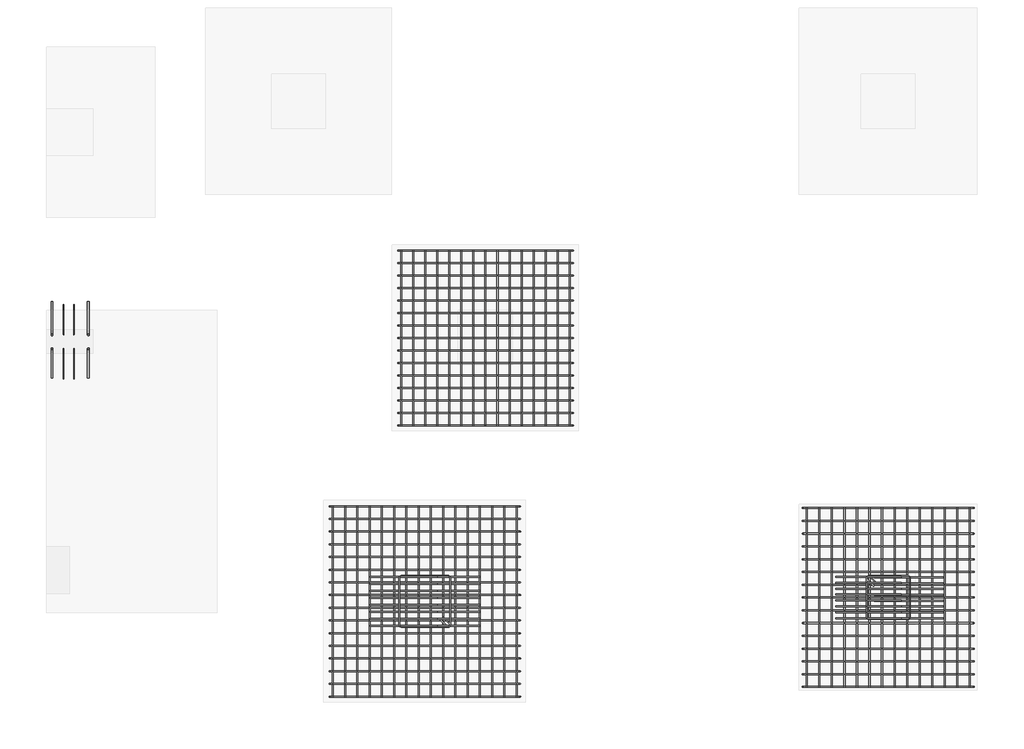
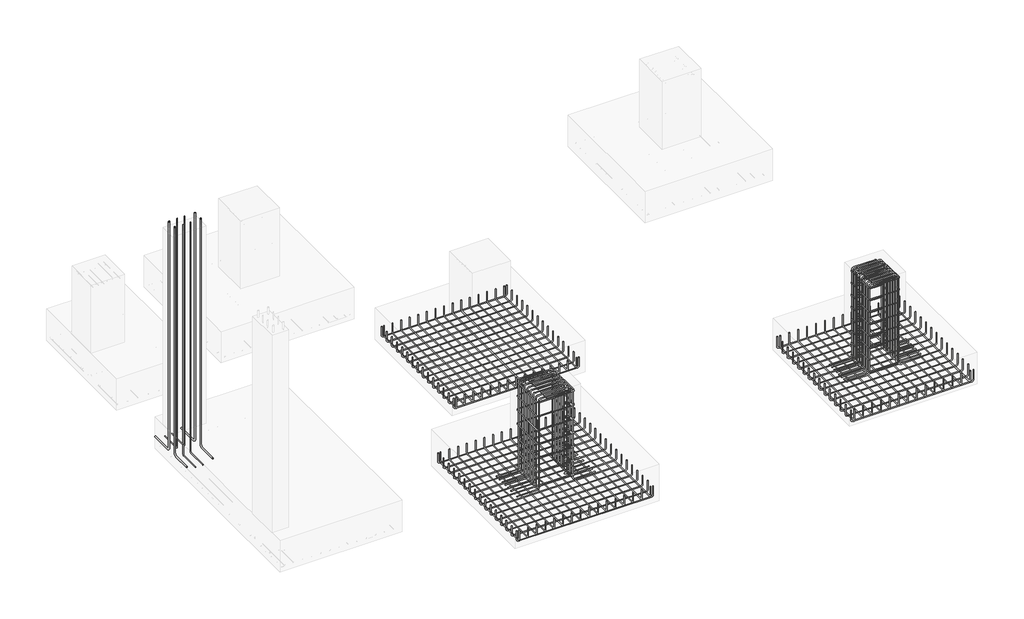
# One storey, part 4 of 6: 16 reinforcing bars.
"""IFC4 building model written with IfcOpenShell, lengths in millimetres."""

from ifc_helpers import new_model, si_unit, point, frame, origin, place, context, project, spatial, polyline, circle_curve, trimmed, segment, composite_curve, source, transform, mapped, element, save
from ifc_brep_helpers import swept_disk

model = new_model("IFC4")

# Units and contexts
model_context = context("Model", 3, world=origin())
ifc_project = project(units=[si_unit("LENGTHUNIT", "METRE", prefix="MILLI")], contexts=[model_context])

# Site, building, storey
site = spatial("IfcSite", under=ifc_project)
building = spatial("IfcBuilding", under=site)
storey = spatial("IfcBuildingStorey", under=building, Elevation=0.0)

# Reinforcing bars
placement = place(None, origin())
reinforcing_bar_shape = source(origin(), model_context, "Body", "SolidModel", [
    swept_disk(composite_curve([segment(polyline([(157700.823207, -99129.4007776, -254.8), (157700.823207, -99129.4007776, -397.2)]), True, "CONTINUOUS"), segment(trimmed(circle_curve(frame((157725.823207, -99129.4007776, -397.2), z_axis=(0.0, -1.0, 0.0), x_axis=(-25.0, 0.0, 0.0)), 25.0), [point((157700.823207, -99129.4007776, -397.2))], [point((157725.823207, -99129.4007776, -422.2))], True, "CARTESIAN"), True, "CONTINUOUS"), segment(polyline([(157725.823207, -99129.4007776, -422.2), (159358.423207, -99129.4007776, -422.2)]), True, "CONTINUOUS"), segment(trimmed(circle_curve(frame((159358.423207, -99129.4007776, -397.2), z_axis=(0.0, -1.0, 0.0), x_axis=(0.0, 0.0, -25.0)), 25.0), [point((159358.423207, -99129.4007776, -422.2))], [point((159383.423207, -99129.4007776, -397.2))], True, "CARTESIAN"), True, "CONTINUOUS"), segment(polyline([(159383.423207, -99129.4007776, -397.2), (159383.423207, -99129.4007776, -254.8)]), True, "CONTINUOUS")], self_intersect=False), 5.0),
])
element("IfcReinforcingBar", 1, at=placement, inside=storey, context=model_context, shape_type="MappedRepresentation", body=[
    mapped(reinforcing_bar_shape, transform((0.0, 0.0, 0.0), x_axis=(1.0, 0.0, 0.0), y_axis=(0.0, 1.0, 0.0), z_axis=(0.0, 0.0, 1.0))),
    mapped(reinforcing_bar_shape, transform((0.0, -125.6285714, 0.0), x_axis=(1.0, 0.0, 0.0), y_axis=(0.0, 1.0, 0.0), z_axis=(0.0, 0.0, 1.0))),
    mapped(reinforcing_bar_shape, transform((0.0, -251.2571429, 0.0), x_axis=(1.0, 0.0, 0.0), y_axis=(0.0, 1.0, 0.0), z_axis=(0.0, 0.0, 1.0))),
    mapped(reinforcing_bar_shape, transform((0.0, -376.8857143, 0.0), x_axis=(1.0, 0.0, 0.0), y_axis=(0.0, 1.0, 0.0), z_axis=(0.0, 0.0, 1.0))),
    mapped(reinforcing_bar_shape, transform((0.0, -502.5142857, 0.0), x_axis=(1.0, 0.0, 0.0), y_axis=(0.0, 1.0, 0.0), z_axis=(0.0, 0.0, 1.0))),
    mapped(reinforcing_bar_shape, transform((0.0, -628.1428571, 0.0), x_axis=(1.0, 0.0, 0.0), y_axis=(0.0, 1.0, 0.0), z_axis=(0.0, 0.0, 1.0))),
    mapped(reinforcing_bar_shape, transform((0.0, -753.7714286, 0.0), x_axis=(1.0, 0.0, 0.0), y_axis=(0.0, 1.0, 0.0), z_axis=(0.0, 0.0, 1.0))),
    mapped(reinforcing_bar_shape, transform((0.0, -879.4, 0.0), x_axis=(1.0, 0.0, 0.0), y_axis=(0.0, 1.0, 0.0), z_axis=(0.0, 0.0, 1.0))),
    mapped(reinforcing_bar_shape, transform((0.0, -1005.0285714, 0.0), x_axis=(1.0, 0.0, 0.0), y_axis=(0.0, 1.0, 0.0), z_axis=(0.0, 0.0, 1.0))),
    mapped(reinforcing_bar_shape, transform((0.0, -1130.6571429, 0.0), x_axis=(1.0, 0.0, 0.0), y_axis=(0.0, 1.0, 0.0), z_axis=(0.0, 0.0, 1.0))),
    mapped(reinforcing_bar_shape, transform((0.0, -1256.2857143, 0.0), x_axis=(1.0, 0.0, 0.0), y_axis=(0.0, 1.0, 0.0), z_axis=(0.0, 0.0, 1.0))),
    mapped(reinforcing_bar_shape, transform((0.0, -1381.9142857, 0.0), x_axis=(1.0, 0.0, 0.0), y_axis=(0.0, 1.0, 0.0), z_axis=(0.0, 0.0, 1.0))),
    mapped(reinforcing_bar_shape, transform((0.0, -1507.5428571, 0.0), x_axis=(1.0, 0.0, 0.0), y_axis=(0.0, 1.0, 0.0), z_axis=(0.0, 0.0, 1.0))),
    mapped(reinforcing_bar_shape, transform((0.0, -1633.1714286, 0.0), x_axis=(1.0, 0.0, 0.0), y_axis=(0.0, 1.0, 0.0), z_axis=(0.0, 0.0, 1.0))),
    mapped(reinforcing_bar_shape, transform((0.0, -1758.8, 0.0), x_axis=(1.0, 0.0, 0.0), y_axis=(0.0, 1.0, 0.0), z_axis=(0.0, 0.0, 1.0))),
])
reinforcing_bar_2_shape = source(origin(), model_context, "Body", "SolidModel", [
    swept_disk(composite_curve([segment(polyline([(157743.6569426, -100888.2007776, -254.8), (157743.6569426, -100888.2007776, -397.2)]), True, "CONTINUOUS"), segment(trimmed(circle_curve(frame((157743.6569426, -100863.2007776, -397.2), z_axis=(1.0, 0.0, 0.0), x_axis=(0.0, -25.0, 0.0)), 25.0), [point((157743.6569426, -100888.2007776, -397.2))], [point((157743.6569426, -100863.2007776, -422.2))], True, "CARTESIAN"), True, "CONTINUOUS"), segment(polyline([(157743.6569426, -100863.2007776, -422.2), (157743.6569426, -99154.4007776, -422.2)]), True, "CONTINUOUS"), segment(trimmed(circle_curve(frame((157743.6569426, -99154.4007776, -397.2), z_axis=(1.0, 0.0, 0.0), x_axis=(0.0, 0.0, -25.0)), 25.0), [point((157743.6569426, -99154.4007776, -422.2))], [point((157743.6569426, -99129.4007776, -397.2))], True, "CARTESIAN"), True, "CONTINUOUS"), segment(polyline([(157743.6569426, -99129.4007776, -397.2), (157743.6569426, -99129.4007776, -254.8)]), True, "CONTINUOUS")], self_intersect=False), 5.0),
])
element("IfcReinforcingBar", 2, at=placement, inside=storey, context=model_context, shape_type="MappedRepresentation", body=[
    mapped(reinforcing_bar_2_shape, transform((0.0, 0.0, 0.0), x_axis=(1.0, 0.0, 0.0), y_axis=(0.0, 1.0, 0.0), z_axis=(0.0, 0.0, 1.0))),
    mapped(reinforcing_bar_2_shape, transform((122.8370266, 0.0, 0.0), x_axis=(1.0, 0.0, 0.0), y_axis=(0.0, 1.0, 0.0), z_axis=(0.0, 0.0, 1.0))),
    mapped(reinforcing_bar_2_shape, transform((245.6740532, 0.0, 0.0), x_axis=(1.0, 0.0, 0.0), y_axis=(0.0, 1.0, 0.0), z_axis=(0.0, 0.0, 1.0))),
    mapped(reinforcing_bar_2_shape, transform((368.5110799, 0.0, 0.0), x_axis=(1.0, 0.0, 0.0), y_axis=(0.0, 1.0, 0.0), z_axis=(0.0, 0.0, 1.0))),
    mapped(reinforcing_bar_2_shape, transform((491.3481065, 0.0, 0.0), x_axis=(1.0, 0.0, 0.0), y_axis=(0.0, 1.0, 0.0), z_axis=(0.0, 0.0, 1.0))),
    mapped(reinforcing_bar_2_shape, transform((614.1851331, 0.0, 0.0), x_axis=(1.0, 0.0, 0.0), y_axis=(0.0, 1.0, 0.0), z_axis=(0.0, 0.0, 1.0))),
    mapped(reinforcing_bar_2_shape, transform((737.0221597, 0.0, 0.0), x_axis=(1.0, 0.0, 0.0), y_axis=(0.0, 1.0, 0.0), z_axis=(0.0, 0.0, 1.0))),
    mapped(reinforcing_bar_2_shape, transform((859.8591864, 0.0, 0.0), x_axis=(1.0, 0.0, 0.0), y_axis=(0.0, 1.0, 0.0), z_axis=(0.0, 0.0, 1.0))),
    mapped(reinforcing_bar_2_shape, transform((982.696213, 0.0, 0.0), x_axis=(1.0, 0.0, 0.0), y_axis=(0.0, 1.0, 0.0), z_axis=(0.0, 0.0, 1.0))),
    mapped(reinforcing_bar_2_shape, transform((1105.5332396, 0.0, 0.0), x_axis=(1.0, 0.0, 0.0), y_axis=(0.0, 1.0, 0.0), z_axis=(0.0, 0.0, 1.0))),
    mapped(reinforcing_bar_2_shape, transform((1228.3702662, 0.0, 0.0), x_axis=(1.0, 0.0, 0.0), y_axis=(0.0, 1.0, 0.0), z_axis=(0.0, 0.0, 1.0))),
    mapped(reinforcing_bar_2_shape, transform((1351.2072929, 0.0, 0.0), x_axis=(1.0, 0.0, 0.0), y_axis=(0.0, 1.0, 0.0), z_axis=(0.0, 0.0, 1.0))),
    mapped(reinforcing_bar_2_shape, transform((1474.0443195, 0.0, 0.0), x_axis=(1.0, 0.0, 0.0), y_axis=(0.0, 1.0, 0.0), z_axis=(0.0, 0.0, 1.0))),
    mapped(reinforcing_bar_2_shape, transform((1596.8813461, 0.0, 0.0), x_axis=(1.0, 0.0, 0.0), y_axis=(0.0, 1.0, 0.0), z_axis=(0.0, 0.0, 1.0))),
])
reinforcing_bar_3_shape = source(origin(), model_context, "Body", "SolidModel", [
    swept_disk(composite_curve([segment(polyline([(153726.0805846, -96596.7317834, -254.8), (153726.0805846, -96596.7317834, -377.2)]), True, "CONTINUOUS"), segment(trimmed(circle_curve(frame((153751.0805846, -96596.7317834, -377.2), z_axis=(0.0, -1.0, 0.0), x_axis=(-25.0, 0.0, 0.0)), 25.0), [point((153726.0805846, -96596.7317834, -377.2))], [point((153751.0805846, -96596.7317834, -402.2))], True, "CARTESIAN"), True, "CONTINUOUS"), segment(polyline([(153751.0805846, -96596.7317834, -402.2), (155419.8805846, -96596.7317834, -402.2)]), True, "CONTINUOUS"), segment(trimmed(circle_curve(frame((155419.8805846, -96596.7317834, -377.2), z_axis=(0.0, -1.0, 0.0), x_axis=(0.0, 0.0, -25.0)), 25.0), [point((155419.8805846, -96596.7317834, -402.2))], [point((155444.8805846, -96596.7317834, -377.2))], True, "CARTESIAN"), True, "CONTINUOUS"), segment(polyline([(155444.8805846, -96596.7317834, -377.2), (155444.8805846, -96596.7317834, -254.8)]), True, "CONTINUOUS")], self_intersect=False), 5.0),
])
element("IfcReinforcingBar", 3, at=placement, inside=storey, context=model_context, shape_type="MappedRepresentation", body=[
    mapped(reinforcing_bar_3_shape, transform((0.0, 0.0, 0.0), x_axis=(1.0, 0.0, 0.0), y_axis=(0.0, 1.0, 0.0), z_axis=(0.0, 0.0, 1.0))),
    mapped(reinforcing_bar_3_shape, transform((0.0, -122.7714286, 0.0), x_axis=(1.0, 0.0, 0.0), y_axis=(0.0, 1.0, 0.0), z_axis=(0.0, 0.0, 1.0))),
    mapped(reinforcing_bar_3_shape, transform((0.0, -245.5428571, 0.0), x_axis=(1.0, 0.0, 0.0), y_axis=(0.0, 1.0, 0.0), z_axis=(0.0, 0.0, 1.0))),
    mapped(reinforcing_bar_3_shape, transform((0.0, -368.3142857, 0.0), x_axis=(1.0, 0.0, 0.0), y_axis=(0.0, 1.0, 0.0), z_axis=(0.0, 0.0, 1.0))),
    mapped(reinforcing_bar_3_shape, transform((0.0, -491.0857143, 0.0), x_axis=(1.0, 0.0, 0.0), y_axis=(0.0, 1.0, 0.0), z_axis=(0.0, 0.0, 1.0))),
    mapped(reinforcing_bar_3_shape, transform((0.0, -613.8571429, 0.0), x_axis=(1.0, 0.0, 0.0), y_axis=(0.0, 1.0, 0.0), z_axis=(0.0, 0.0, 1.0))),
    mapped(reinforcing_bar_3_shape, transform((0.0, -736.6285714, 0.0), x_axis=(1.0, 0.0, 0.0), y_axis=(0.0, 1.0, 0.0), z_axis=(0.0, 0.0, 1.0))),
    mapped(reinforcing_bar_3_shape, transform((0.0, -859.4, 0.0), x_axis=(1.0, 0.0, 0.0), y_axis=(0.0, 1.0, 0.0), z_axis=(0.0, 0.0, 1.0))),
    mapped(reinforcing_bar_3_shape, transform((0.0, -982.1714286, 0.0), x_axis=(1.0, 0.0, 0.0), y_axis=(0.0, 1.0, 0.0), z_axis=(0.0, 0.0, 1.0))),
    mapped(reinforcing_bar_3_shape, transform((0.0, -1104.9428571, 0.0), x_axis=(1.0, 0.0, 0.0), y_axis=(0.0, 1.0, 0.0), z_axis=(0.0, 0.0, 1.0))),
    mapped(reinforcing_bar_3_shape, transform((0.0, -1227.7142857, 0.0), x_axis=(1.0, 0.0, 0.0), y_axis=(0.0, 1.0, 0.0), z_axis=(0.0, 0.0, 1.0))),
    mapped(reinforcing_bar_3_shape, transform((0.0, -1350.4857143, 0.0), x_axis=(1.0, 0.0, 0.0), y_axis=(0.0, 1.0, 0.0), z_axis=(0.0, 0.0, 1.0))),
    mapped(reinforcing_bar_3_shape, transform((0.0, -1473.2571429, 0.0), x_axis=(1.0, 0.0, 0.0), y_axis=(0.0, 1.0, 0.0), z_axis=(0.0, 0.0, 1.0))),
    mapped(reinforcing_bar_3_shape, transform((0.0, -1596.0285714, 0.0), x_axis=(1.0, 0.0, 0.0), y_axis=(0.0, 1.0, 0.0), z_axis=(0.0, 0.0, 1.0))),
    mapped(reinforcing_bar_3_shape, transform((0.0, -1718.8, 0.0), x_axis=(1.0, 0.0, 0.0), y_axis=(0.0, 1.0, 0.0), z_axis=(0.0, 0.0, 1.0))),
])
reinforcing_bar_4_shape = source(origin(), model_context, "Body", "SolidModel", [
    swept_disk(composite_curve([segment(polyline([(153758.096494, -98315.5317834, -254.8), (153758.096494, -98315.5317834, -377.2)]), True, "CONTINUOUS"), segment(trimmed(circle_curve(frame((153758.096494, -98290.5317834, -377.2), z_axis=(1.0, 0.0, 0.0), x_axis=(0.0, -25.0, 0.0)), 25.0), [point((153758.096494, -98315.5317834, -377.2))], [point((153758.096494, -98290.5317834, -402.2))], True, "CARTESIAN"), True, "CONTINUOUS"), segment(polyline([(153758.096494, -98290.5317834, -402.2), (153758.096494, -96621.7317834, -402.2)]), True, "CONTINUOUS"), segment(trimmed(circle_curve(frame((153758.096494, -96621.7317834, -377.2), z_axis=(1.0, 0.0, 0.0), x_axis=(0.0, 0.0, -25.0)), 25.0), [point((153758.096494, -96621.7317834, -402.2))], [point((153758.096494, -96596.7317834, -377.2))], True, "CARTESIAN"), True, "CONTINUOUS"), segment(polyline([(153758.096494, -96596.7317834, -377.2), (153758.096494, -96596.7317834, -254.8)]), True, "CONTINUOUS")], self_intersect=False), 5.0),
])
element("IfcReinforcingBar", 4, at=placement, inside=storey, context=model_context, shape_type="MappedRepresentation", body=[
    mapped(reinforcing_bar_4_shape, transform((0.0, 0.0, 0.0), x_axis=(1.0, 0.0, 0.0), y_axis=(0.0, 1.0, 0.0), z_axis=(0.0, 0.0, 1.0))),
    mapped(reinforcing_bar_4_shape, transform((118.1173845, 0.0, 0.0), x_axis=(1.0, 0.0, 0.0), y_axis=(0.0, 1.0, 0.0), z_axis=(0.0, 0.0, 1.0))),
    mapped(reinforcing_bar_4_shape, transform((236.2347691, 0.0, 0.0), x_axis=(1.0, 0.0, 0.0), y_axis=(0.0, 1.0, 0.0), z_axis=(0.0, 0.0, 1.0))),
    mapped(reinforcing_bar_4_shape, transform((354.3521536, 0.0, 0.0), x_axis=(1.0, 0.0, 0.0), y_axis=(0.0, 1.0, 0.0), z_axis=(0.0, 0.0, 1.0))),
    mapped(reinforcing_bar_4_shape, transform((472.4695381, 0.0, 0.0), x_axis=(1.0, 0.0, 0.0), y_axis=(0.0, 1.0, 0.0), z_axis=(0.0, 0.0, 1.0))),
    mapped(reinforcing_bar_4_shape, transform((590.5869227, 0.0, 0.0), x_axis=(1.0, 0.0, 0.0), y_axis=(0.0, 1.0, 0.0), z_axis=(0.0, 0.0, 1.0))),
    mapped(reinforcing_bar_4_shape, transform((708.7043072, 0.0, 0.0), x_axis=(1.0, 0.0, 0.0), y_axis=(0.0, 1.0, 0.0), z_axis=(0.0, 0.0, 1.0))),
    mapped(reinforcing_bar_4_shape, transform((826.8216917, 0.0, 0.0), x_axis=(1.0, 0.0, 0.0), y_axis=(0.0, 1.0, 0.0), z_axis=(0.0, 0.0, 1.0))),
    mapped(reinforcing_bar_4_shape, transform((944.9390763, 0.0, 0.0), x_axis=(1.0, 0.0, 0.0), y_axis=(0.0, 1.0, 0.0), z_axis=(0.0, 0.0, 1.0))),
    mapped(reinforcing_bar_4_shape, transform((1063.0564608, 0.0, 0.0), x_axis=(1.0, 0.0, 0.0), y_axis=(0.0, 1.0, 0.0), z_axis=(0.0, 0.0, 1.0))),
    mapped(reinforcing_bar_4_shape, transform((1181.1738453, 0.0, 0.0), x_axis=(1.0, 0.0, 0.0), y_axis=(0.0, 1.0, 0.0), z_axis=(0.0, 0.0, 1.0))),
    mapped(reinforcing_bar_4_shape, transform((1299.2912299, 0.0, 0.0), x_axis=(1.0, 0.0, 0.0), y_axis=(0.0, 1.0, 0.0), z_axis=(0.0, 0.0, 1.0))),
    mapped(reinforcing_bar_4_shape, transform((1417.4086144, 0.0, 0.0), x_axis=(1.0, 0.0, 0.0), y_axis=(0.0, 1.0, 0.0), z_axis=(0.0, 0.0, 1.0))),
    mapped(reinforcing_bar_4_shape, transform((1535.5259989, 0.0, 0.0), x_axis=(1.0, 0.0, 0.0), y_axis=(0.0, 1.0, 0.0), z_axis=(0.0, 0.0, 1.0))),
    mapped(reinforcing_bar_4_shape, transform((1653.6433835, 0.0, 0.0), x_axis=(1.0, 0.0, 0.0), y_axis=(0.0, 1.0, 0.0), z_axis=(0.0, 0.0, 1.0))),
])
reinforcing_bar_5_shape = source(origin(), model_context, "Body", "SolidModel", [
    swept_disk(composite_curve([segment(polyline([(153052.9805846, -99111.3007776, -331.0), (153052.9805846, -99111.3007776, -453.4)]), True, "CONTINUOUS"), segment(trimmed(circle_curve(frame((153077.9805846, -99111.3007776, -453.4), z_axis=(0.0, -1.0, 0.0), x_axis=(-25.0, 0.0, 0.0)), 25.0), [point((153052.9805846, -99111.3007776, -453.4))], [point((153077.9805846, -99111.3007776, -478.4))], True, "CARTESIAN"), True, "CONTINUOUS"), segment(polyline([(153077.9805846, -99111.3007776, -478.4), (154899.1805846, -99111.3007776, -478.4)]), True, "CONTINUOUS"), segment(trimmed(circle_curve(frame((154899.1805846, -99111.3007776, -453.4), z_axis=(0.0, -1.0, 0.0), x_axis=(0.0, 0.0, -25.0)), 25.0), [point((154899.1805846, -99111.3007776, -478.4))], [point((154924.1805846, -99111.3007776, -453.4))], True, "CARTESIAN"), True, "CONTINUOUS"), segment(polyline([(154924.1805846, -99111.3007776, -453.4), (154924.1805846, -99111.3007776, -331.0)]), True, "CONTINUOUS")], self_intersect=False), 5.0),
])
element("IfcReinforcingBar", 5, at=placement, inside=storey, context=model_context, shape_type="MappedRepresentation", body=[
    mapped(reinforcing_bar_5_shape, transform((0.0, 0.0, 0.0), x_axis=(1.0, 0.0, 0.0), y_axis=(0.0, 1.0, 0.0), z_axis=(0.0, 0.0, 1.0))),
    mapped(reinforcing_bar_5_shape, transform((0.0, -124.7466667, 0.0), x_axis=(1.0, 0.0, 0.0), y_axis=(0.0, 1.0, 0.0), z_axis=(0.0, 0.0, 1.0))),
    mapped(reinforcing_bar_5_shape, transform((0.0, -249.4933333, 0.0), x_axis=(1.0, 0.0, 0.0), y_axis=(0.0, 1.0, 0.0), z_axis=(0.0, 0.0, 1.0))),
    mapped(reinforcing_bar_5_shape, transform((0.0, -374.24, 0.0), x_axis=(1.0, 0.0, 0.0), y_axis=(0.0, 1.0, 0.0), z_axis=(0.0, 0.0, 1.0))),
    mapped(reinforcing_bar_5_shape, transform((0.0, -498.9866667, 0.0), x_axis=(1.0, 0.0, 0.0), y_axis=(0.0, 1.0, 0.0), z_axis=(0.0, 0.0, 1.0))),
    mapped(reinforcing_bar_5_shape, transform((0.0, -623.7333333, 0.0), x_axis=(1.0, 0.0, 0.0), y_axis=(0.0, 1.0, 0.0), z_axis=(0.0, 0.0, 1.0))),
    mapped(reinforcing_bar_5_shape, transform((0.0, -748.48, 0.0), x_axis=(1.0, 0.0, 0.0), y_axis=(0.0, 1.0, 0.0), z_axis=(0.0, 0.0, 1.0))),
    mapped(reinforcing_bar_5_shape, transform((0.0, -873.2266667, 0.0), x_axis=(1.0, 0.0, 0.0), y_axis=(0.0, 1.0, 0.0), z_axis=(0.0, 0.0, 1.0))),
    mapped(reinforcing_bar_5_shape, transform((0.0, -997.9733333, 0.0), x_axis=(1.0, 0.0, 0.0), y_axis=(0.0, 1.0, 0.0), z_axis=(0.0, 0.0, 1.0))),
    mapped(reinforcing_bar_5_shape, transform((0.0, -1122.72, 0.0), x_axis=(1.0, 0.0, 0.0), y_axis=(0.0, 1.0, 0.0), z_axis=(0.0, 0.0, 1.0))),
    mapped(reinforcing_bar_5_shape, transform((0.0, -1247.4666667, 0.0), x_axis=(1.0, 0.0, 0.0), y_axis=(0.0, 1.0, 0.0), z_axis=(0.0, 0.0, 1.0))),
    mapped(reinforcing_bar_5_shape, transform((0.0, -1372.2133333, 0.0), x_axis=(1.0, 0.0, 0.0), y_axis=(0.0, 1.0, 0.0), z_axis=(0.0, 0.0, 1.0))),
    mapped(reinforcing_bar_5_shape, transform((0.0, -1496.96, 0.0), x_axis=(1.0, 0.0, 0.0), y_axis=(0.0, 1.0, 0.0), z_axis=(0.0, 0.0, 1.0))),
    mapped(reinforcing_bar_5_shape, transform((0.0, -1621.7066667, 0.0), x_axis=(1.0, 0.0, 0.0), y_axis=(0.0, 1.0, 0.0), z_axis=(0.0, 0.0, 1.0))),
    mapped(reinforcing_bar_5_shape, transform((0.0, -1746.4533333, 0.0), x_axis=(1.0, 0.0, 0.0), y_axis=(0.0, 1.0, 0.0), z_axis=(0.0, 0.0, 1.0))),
    mapped(reinforcing_bar_5_shape, transform((0.0, -1871.2, 0.0), x_axis=(1.0, 0.0, 0.0), y_axis=(0.0, 1.0, 0.0), z_axis=(0.0, 0.0, 1.0))),
])
reinforcing_bar_6_shape = source(origin(), model_context, "Body", "SolidModel", [
    swept_disk(composite_curve([segment(polyline([(153084.996494, -100982.5007776, -331.0), (153084.996494, -100982.5007776, -453.4)]), True, "CONTINUOUS"), segment(trimmed(circle_curve(frame((153084.996494, -100957.5007776, -453.4), z_axis=(1.0, 0.0, 0.0), x_axis=(0.0, -25.0, 0.0)), 25.0), [point((153084.996494, -100982.5007776, -453.4))], [point((153084.996494, -100957.5007776, -478.4))], True, "CARTESIAN"), True, "CONTINUOUS"), segment(polyline([(153084.996494, -100957.5007776, -478.4), (153084.996494, -99136.3007776, -478.4)]), True, "CONTINUOUS"), segment(trimmed(circle_curve(frame((153084.996494, -99136.3007776, -453.4), z_axis=(1.0, 0.0, 0.0), x_axis=(0.0, 0.0, -25.0)), 25.0), [point((153084.996494, -99136.3007776, -478.4))], [point((153084.996494, -99111.3007776, -453.4))], True, "CARTESIAN"), True, "CONTINUOUS"), segment(polyline([(153084.996494, -99111.3007776, -453.4), (153084.996494, -99111.3007776, -331.0)]), True, "CONTINUOUS")], self_intersect=False), 5.0),
])
element("IfcReinforcingBar", 6, at=placement, inside=storey, context=model_context, shape_type="MappedRepresentation", body=[
    mapped(reinforcing_bar_6_shape, transform((0.0, 0.0, 0.0), x_axis=(1.0, 0.0, 0.0), y_axis=(0.0, 1.0, 0.0), z_axis=(0.0, 0.0, 1.0))),
    mapped(reinforcing_bar_6_shape, transform((120.4028922, 0.0, 0.0), x_axis=(1.0, 0.0, 0.0), y_axis=(0.0, 1.0, 0.0), z_axis=(0.0, 0.0, 1.0))),
    mapped(reinforcing_bar_6_shape, transform((240.8057845, 0.0, 0.0), x_axis=(1.0, 0.0, 0.0), y_axis=(0.0, 1.0, 0.0), z_axis=(0.0, 0.0, 1.0))),
    mapped(reinforcing_bar_6_shape, transform((361.2086767, 0.0, 0.0), x_axis=(1.0, 0.0, 0.0), y_axis=(0.0, 1.0, 0.0), z_axis=(0.0, 0.0, 1.0))),
    mapped(reinforcing_bar_6_shape, transform((481.6115689, 0.0, 0.0), x_axis=(1.0, 0.0, 0.0), y_axis=(0.0, 1.0, 0.0), z_axis=(0.0, 0.0, 1.0))),
    mapped(reinforcing_bar_6_shape, transform((602.0144612, 0.0, 0.0), x_axis=(1.0, 0.0, 0.0), y_axis=(0.0, 1.0, 0.0), z_axis=(0.0, 0.0, 1.0))),
    mapped(reinforcing_bar_6_shape, transform((722.4173534, 0.0, 0.0), x_axis=(1.0, 0.0, 0.0), y_axis=(0.0, 1.0, 0.0), z_axis=(0.0, 0.0, 1.0))),
    mapped(reinforcing_bar_6_shape, transform((842.8202456, 0.0, 0.0), x_axis=(1.0, 0.0, 0.0), y_axis=(0.0, 1.0, 0.0), z_axis=(0.0, 0.0, 1.0))),
    mapped(reinforcing_bar_6_shape, transform((963.2231378, 0.0, 0.0), x_axis=(1.0, 0.0, 0.0), y_axis=(0.0, 1.0, 0.0), z_axis=(0.0, 0.0, 1.0))),
    mapped(reinforcing_bar_6_shape, transform((1083.6260301, 0.0, 0.0), x_axis=(1.0, 0.0, 0.0), y_axis=(0.0, 1.0, 0.0), z_axis=(0.0, 0.0, 1.0))),
    mapped(reinforcing_bar_6_shape, transform((1204.0289223, 0.0, 0.0), x_axis=(1.0, 0.0, 0.0), y_axis=(0.0, 1.0, 0.0), z_axis=(0.0, 0.0, 1.0))),
    mapped(reinforcing_bar_6_shape, transform((1324.4318145, 0.0, 0.0), x_axis=(1.0, 0.0, 0.0), y_axis=(0.0, 1.0, 0.0), z_axis=(0.0, 0.0, 1.0))),
    mapped(reinforcing_bar_6_shape, transform((1444.8347068, 0.0, 0.0), x_axis=(1.0, 0.0, 0.0), y_axis=(0.0, 1.0, 0.0), z_axis=(0.0, 0.0, 1.0))),
    mapped(reinforcing_bar_6_shape, transform((1565.237599, 0.0, 0.0), x_axis=(1.0, 0.0, 0.0), y_axis=(0.0, 1.0, 0.0), z_axis=(0.0, 0.0, 1.0))),
    mapped(reinforcing_bar_6_shape, transform((1685.6404912, 0.0, 0.0), x_axis=(1.0, 0.0, 0.0), y_axis=(0.0, 1.0, 0.0), z_axis=(0.0, 0.0, 1.0))),
    mapped(reinforcing_bar_6_shape, transform((1806.0433835, 0.0, 0.0), x_axis=(1.0, 0.0, 0.0), y_axis=(0.0, 1.0, 0.0), z_axis=(0.0, 0.0, 1.0))),
])
reinforcing_bar_7_shape = source(origin(), model_context, "Body", "SolidModel", [
    swept_disk(composite_curve([segment(polyline([(158669.5918058, -99805.1007776, 933.0070241), (158366.598207, -99805.1007776, 933.0070241)]), True, "CONTINUOUS"), segment(trimmed(circle_curve(frame((158366.598207, -99805.1007776, 908.0070241), z_axis=(0.0, -1.0, 0.0), x_axis=(0.0, 0.0, 25.0)), 25.0), [point((158366.598207, -99805.1007776, 933.0070241))], [point((158341.598207, -99805.1007776, 908.0070241))], True, "CARTESIAN"), True, "CONTINUOUS"), segment(polyline([(158341.598207, -99805.1007776, 908.0070241), (158341.598207, -99805.1007776, -343.6790158)]), True, "CONTINUOUS"), segment(trimmed(circle_curve(frame((158316.598207, -99805.1007776, -343.6790158), z_axis=(0.0, 1.0, 0.0), x_axis=(25.0, 0.0, 0.0)), 25.0), [point((158341.598207, -99805.1007776, -343.6790158))], [point((158316.598207, -99805.1007776, -368.6790158))], True, "CARTESIAN"), True, "CONTINUOUS"), segment(polyline([(158316.598207, -99805.1007776, -368.6790158), (158027.6032021, -99805.1007776, -368.6790158)]), True, "CONTINUOUS")], self_intersect=False), 5.0),
])
element("IfcReinforcingBar", 7, at=placement, inside=storey, context=model_context, shape_type="MappedRepresentation", body=[
    mapped(reinforcing_bar_7_shape, transform((0.0, 0.0, 0.0), x_axis=(1.0, 0.0, 0.0), y_axis=(0.0, 1.0, 0.0), z_axis=(0.0, 0.0, 1.0))),
    mapped(reinforcing_bar_7_shape, transform((0.0, -58.2, 0.0), x_axis=(1.0, 0.0, 0.0), y_axis=(0.0, 1.0, 0.0), z_axis=(0.0, 0.0, 1.0))),
    mapped(reinforcing_bar_7_shape, transform((0.0, -116.4, 0.0), x_axis=(1.0, 0.0, 0.0), y_axis=(0.0, 1.0, 0.0), z_axis=(0.0, 0.0, 1.0))),
    mapped(reinforcing_bar_7_shape, transform((0.0, -174.6, 0.0), x_axis=(1.0, 0.0, 0.0), y_axis=(0.0, 1.0, 0.0), z_axis=(0.0, 0.0, 1.0))),
    mapped(reinforcing_bar_7_shape, transform((0.0, -232.8, 0.0), x_axis=(1.0, 0.0, 0.0), y_axis=(0.0, 1.0, 0.0), z_axis=(0.0, 0.0, 1.0))),
    mapped(reinforcing_bar_7_shape, transform((0.0, -291.0, 0.0), x_axis=(1.0, 0.0, 0.0), y_axis=(0.0, 1.0, 0.0), z_axis=(0.0, 0.0, 1.0))),
    mapped(reinforcing_bar_7_shape, transform((0.0, -349.2, 0.0), x_axis=(1.0, 0.0, 0.0), y_axis=(0.0, 1.0, 0.0), z_axis=(0.0, 0.0, 1.0))),
    mapped(reinforcing_bar_7_shape, transform((0.0, -407.4, 0.0), x_axis=(1.0, 0.0, 0.0), y_axis=(0.0, 1.0, 0.0), z_axis=(0.0, 0.0, 1.0))),
])
reinforcing_bar_8_shape = source(origin(), model_context, "Body", "SolidModel", [
    swept_disk(composite_curve([segment(polyline([(158403.7180958, -100212.5007776, 915.0304286), (158719.235707, -100212.5007776, 915.0304286)]), True, "CONTINUOUS"), segment(trimmed(circle_curve(frame((158719.235707, -100212.5007776, 890.0304286), z_axis=(0.0, 1.0, 0.0), x_axis=(0.0, 0.0, 25.0)), 25.0), [point((158719.235707, -100212.5007776, 915.0304286))], [point((158744.235707, -100212.5007776, 890.0304286))], True, "CARTESIAN"), True, "CONTINUOUS"), segment(polyline([(158744.235707, -100212.5007776, 890.0304286), (158744.235707, -100212.5007776, -342.7230591)]), True, "CONTINUOUS"), segment(trimmed(circle_curve(frame((158769.235707, -100212.5007776, -342.7230591), z_axis=(0.0, -1.0, 0.0), x_axis=(-25.0, 0.0, 0.0)), 25.0), [point((158744.235707, -100212.5007776, -342.7230591))], [point((158769.235707, -100212.5007776, -367.7230591))], True, "CARTESIAN"), True, "CONTINUOUS"), segment(polyline([(158769.235707, -100212.5007776, -367.7230591), (159082.1226497, -100212.5007776, -367.7230591)]), True, "CONTINUOUS")], self_intersect=False), 5.0),
])
element("IfcReinforcingBar", 8, at=placement, inside=storey, context=model_context, shape_type="MappedRepresentation", body=[
    mapped(reinforcing_bar_8_shape, transform((0.0, 0.0, 0.0), x_axis=(1.0, 0.0, 0.0), y_axis=(0.0, 1.0, 0.0), z_axis=(0.0, 0.0, 1.0))),
    mapped(reinforcing_bar_8_shape, transform((0.0, 57.5196429, 0.0), x_axis=(1.0, 0.0, 0.0), y_axis=(0.0, 1.0, 0.0), z_axis=(0.0, 0.0, 1.0))),
    mapped(reinforcing_bar_8_shape, transform((0.0, 115.0392857, 0.0), x_axis=(1.0, 0.0, 0.0), y_axis=(0.0, 1.0, 0.0), z_axis=(0.0, 0.0, 1.0))),
    mapped(reinforcing_bar_8_shape, transform((0.0, 172.5589286, 0.0), x_axis=(1.0, 0.0, 0.0), y_axis=(0.0, 1.0, 0.0), z_axis=(0.0, 0.0, 1.0))),
    mapped(reinforcing_bar_8_shape, transform((0.0, 230.0785714, 0.0), x_axis=(1.0, 0.0, 0.0), y_axis=(0.0, 1.0, 0.0), z_axis=(0.0, 0.0, 1.0))),
    mapped(reinforcing_bar_8_shape, transform((0.0, 287.5982143, 0.0), x_axis=(1.0, 0.0, 0.0), y_axis=(0.0, 1.0, 0.0), z_axis=(0.0, 0.0, 1.0))),
    mapped(reinforcing_bar_8_shape, transform((0.0, 345.1178571, 0.0), x_axis=(1.0, 0.0, 0.0), y_axis=(0.0, 1.0, 0.0), z_axis=(0.0, 0.0, 1.0))),
    mapped(reinforcing_bar_8_shape, transform((0.0, 402.6375, 0.0), x_axis=(1.0, 0.0, 0.0), y_axis=(0.0, 1.0, 0.0), z_axis=(0.0, 0.0, 1.0))),
])
reinforcing_bar_9_shape = source(origin(), model_context, "Body", "SolidModel", [
    swept_disk(composite_curve([segment(polyline([(158427.9120597, -99866.305359, -326.840765), (158363.5653426, -99801.958642, -326.840765)]), True, "CONTINUOUS"), segment(trimmed(circle_curve(frame((158349.423207, -99816.1007776, -326.840765), z_axis=(0.0, 0.0, 1.0), x_axis=(14.142135599977337, 14.14213560000644, 0.0)), 20.0), [point((158363.5653426, -99801.958642, -326.840765))], [point((158329.423207, -99816.1007776, -326.840765))], True, "CARTESIAN"), True, "CONTINUOUS"), segment(polyline([(158329.423207, -99816.1007776, -326.840765), (158329.423207, -100201.5007776, -326.840765)]), True, "CONTINUOUS"), segment(trimmed(circle_curve(frame((158349.423207, -100201.5007776, -326.840765), z_axis=(0.0, 0.0, 1.0), x_axis=(-20.0, 0.0, 0.0)), 20.0), [point((158329.423207, -100201.5007776, -326.840765))], [point((158349.423207, -100221.5007776, -326.840765))], True, "CARTESIAN"), True, "CONTINUOUS"), segment(polyline([(158349.423207, -100221.5007776, -326.840765), (158734.823207, -100221.5007776, -326.840765)]), True, "CONTINUOUS"), segment(trimmed(circle_curve(frame((158734.823207, -100201.5043132, -327.2168151), z_axis=(0.0, 0.01880250526134244, 0.9998232172718822), x_axis=(0.0, -19.99646439999924, 0.37605010000004313)), 20.0), [point((158734.823207, -100221.5007776, -326.840765))], [point((158754.823207, -100201.5043132, -327.2168151))], True, "CARTESIAN"), True, "CONTINUOUS"), segment(polyline([(158754.823207, -100201.5043132, -327.2168151), (158754.823207, -99816.0972419, -334.4647149)]), True, "CONTINUOUS"), segment(trimmed(circle_curve(frame((158734.823207, -99816.0972419, -334.4647149), z_axis=(0.0, 0.01880250526134244, 0.9998232172718822), x_axis=(20.0, 0.0, 0.0)), 20.0), [point((158754.823207, -99816.0972419, -334.4647149))], [point((158734.823207, -99796.1007776, -334.840765))], True, "CARTESIAN"), True, "CONTINUOUS"), segment(polyline([(158734.823207, -99796.1007776, -334.840765), (158349.423207, -99796.1007776, -334.840765)]), True, "CONTINUOUS"), segment(trimmed(circle_curve(frame((158349.423207, -99816.1007776, -334.840765), z_axis=(0.0, 0.0, 1.0), x_axis=(0.0, 20.0, 0.0)), 20.0), [point((158349.423207, -99796.1007776, -334.840765))], [point((158335.2810714, -99830.2429132, -334.840765))], True, "CARTESIAN"), True, "CONTINUOUS"), segment(polyline([(158335.2810714, -99830.2429132, -334.840765), (158399.6277885, -99894.5896303, -334.840765)]), True, "CONTINUOUS")], self_intersect=False), 4.0),
])
element("IfcReinforcingBar", 9, at=placement, inside=storey, context=model_context, shape_type="MappedRepresentation", body=[
    mapped(reinforcing_bar_9_shape, transform((0.0, 0.0, 0.0), x_axis=(1.0, 0.0, 0.0), y_axis=(0.0, 1.0, 0.0), z_axis=(0.0, 0.0, 1.0))),
    mapped(reinforcing_bar_9_shape, transform((0.0, 0.0, 174.4633022), x_axis=(1.0, 0.0, 0.0), y_axis=(0.0, 1.0, 0.0), z_axis=(0.0, 0.0, 1.0))),
    mapped(reinforcing_bar_9_shape, transform((0.0, 0.0, 348.9266043), x_axis=(1.0, 0.0, 0.0), y_axis=(0.0, 1.0, 0.0), z_axis=(0.0, 0.0, 1.0))),
    mapped(reinforcing_bar_9_shape, transform((0.0, 0.0, 523.3899065), x_axis=(1.0, 0.0, 0.0), y_axis=(0.0, 1.0, 0.0), z_axis=(0.0, 0.0, 1.0))),
    mapped(reinforcing_bar_9_shape, transform((0.0, 0.0, 697.8532086), x_axis=(1.0, 0.0, 0.0), y_axis=(0.0, 1.0, 0.0), z_axis=(0.0, 0.0, 1.0))),
    mapped(reinforcing_bar_9_shape, transform((0.0, 0.0, 872.3165108), x_axis=(1.0, 0.0, 0.0), y_axis=(0.0, 1.0, 0.0), z_axis=(0.0, 0.0, 1.0))),
    mapped(reinforcing_bar_9_shape, transform((0.0, 0.0, 1046.7798129), x_axis=(1.0, 0.0, 0.0), y_axis=(0.0, 1.0, 0.0), z_axis=(0.0, 0.0, 1.0))),
    mapped(reinforcing_bar_9_shape, transform((0.0, 0.0, 1221.2431151), x_axis=(1.0, 0.0, 0.0), y_axis=(0.0, 1.0, 0.0), z_axis=(0.0, 0.0, 1.0))),
])
reinforcing_bar_10_shape = source(origin(), model_context, "Body", "SolidModel", [
    swept_disk(composite_curve([segment(polyline([(154112.6118405, -99805.1007776, 921.7139079), (153782.0118405, -99805.1007776, 921.7139079)]), True, "CONTINUOUS"), segment(trimmed(circle_curve(frame((153782.0118405, -99805.1007776, 896.7139079), z_axis=(0.0, -1.0, 0.0), x_axis=(0.0, 0.0, 25.0)), 25.0), [point((153782.0118405, -99805.1007776, 921.7139079))], [point((153757.0118405, -99805.1007776, 896.7139079))], True, "CARTESIAN"), True, "CONTINUOUS"), segment(polyline([(153757.0118405, -99805.1007776, 896.7139079), (153757.0118405, -99805.1007776, -364.6745859)]), True, "CONTINUOUS"), segment(trimmed(circle_curve(frame((153732.0118405, -99805.1007776, -364.6745859), z_axis=(0.0, 1.0, 0.0), x_axis=(25.0, 0.0, 0.0)), 25.0), [point((153757.0118405, -99805.1007776, -364.6745859))], [point((153732.0118405, -99805.1007776, -389.6745859))], True, "CARTESIAN"), True, "CONTINUOUS"), segment(polyline([(153732.0118405, -99805.1007776, -389.6745859), (153452.2118405, -99805.1007776, -389.6745859)]), True, "CONTINUOUS")], self_intersect=False), 5.0),
])
element("IfcReinforcingBar", 10, at=placement, inside=storey, context=model_context, shape_type="MappedRepresentation", body=[
    mapped(reinforcing_bar_10_shape, transform((0.0, 0.0, 0.0), x_axis=(1.0, 0.0, 0.0), y_axis=(0.0, 1.0, 0.0), z_axis=(0.0, 0.0, 1.0))),
    mapped(reinforcing_bar_10_shape, transform((0.0, -69.0857143, 0.0), x_axis=(1.0, 0.0, 0.0), y_axis=(0.0, 1.0, 0.0), z_axis=(0.0, 0.0, 1.0))),
    mapped(reinforcing_bar_10_shape, transform((0.0, -138.1714286, 0.0), x_axis=(1.0, 0.0, 0.0), y_axis=(0.0, 1.0, 0.0), z_axis=(0.0, 0.0, 1.0))),
    mapped(reinforcing_bar_10_shape, transform((0.0, -207.2571429, 0.0), x_axis=(1.0, 0.0, 0.0), y_axis=(0.0, 1.0, 0.0), z_axis=(0.0, 0.0, 1.0))),
    mapped(reinforcing_bar_10_shape, transform((0.0, -276.3428571, 0.0), x_axis=(1.0, 0.0, 0.0), y_axis=(0.0, 1.0, 0.0), z_axis=(0.0, 0.0, 1.0))),
    mapped(reinforcing_bar_10_shape, transform((0.0, -345.4285714, 0.0), x_axis=(1.0, 0.0, 0.0), y_axis=(0.0, 1.0, 0.0), z_axis=(0.0, 0.0, 1.0))),
    mapped(reinforcing_bar_10_shape, transform((0.0, -414.5142857, 0.0), x_axis=(1.0, 0.0, 0.0), y_axis=(0.0, 1.0, 0.0), z_axis=(0.0, 0.0, 1.0))),
    mapped(reinforcing_bar_10_shape, transform((0.0, -483.6, 0.0), x_axis=(1.0, 0.0, 0.0), y_axis=(0.0, 1.0, 0.0), z_axis=(0.0, 0.0, 1.0))),
])
reinforcing_bar_11_shape = source(origin(), model_context, "Body", "SolidModel", [
    swept_disk(composite_curve([segment(polyline([(153860.4691314, -100288.7007776, 903.3038035), (154197.4191314, -100288.7007776, 903.3038035)]), True, "CONTINUOUS"), segment(trimmed(circle_curve(frame((154197.4191314, -100288.7007776, 878.3038035), z_axis=(0.0, 1.0, 0.0), x_axis=(0.0, 0.0, 25.0)), 25.0), [point((154197.4191314, -100288.7007776, 903.3038035))], [point((154222.4191314, -100288.7007776, 878.3038035))], True, "CARTESIAN"), True, "CONTINUOUS"), segment(polyline([(154222.4191314, -100288.7007776, 878.3038035), (154222.4191314, -100288.7007776, -381.4407624)]), True, "CONTINUOUS"), segment(trimmed(circle_curve(frame((154247.4191314, -100288.7007776, -381.4407624), z_axis=(0.0, -1.0, 0.0), x_axis=(-25.0, 0.0, 0.0)), 25.0), [point((154222.4191314, -100288.7007776, -381.4407624))], [point((154247.4191314, -100288.7007776, -406.4407624))], True, "CARTESIAN"), True, "CONTINUOUS"), segment(polyline([(154247.4191314, -100288.7007776, -406.4407624), (154527.2191314, -100288.7007776, -406.4407624)]), True, "CONTINUOUS")], self_intersect=False), 5.0),
])
element("IfcReinforcingBar", 11, at=placement, inside=storey, context=model_context, shape_type="MappedRepresentation", body=[
    mapped(reinforcing_bar_11_shape, transform((0.0, 0.0, 0.0), x_axis=(1.0, 0.0, 0.0), y_axis=(0.0, 1.0, 0.0), z_axis=(0.0, 0.0, 1.0))),
    mapped(reinforcing_bar_11_shape, transform((0.0, 69.0857143, 0.0), x_axis=(1.0, 0.0, 0.0), y_axis=(0.0, 1.0, 0.0), z_axis=(0.0, 0.0, 1.0))),
    mapped(reinforcing_bar_11_shape, transform((0.0, 138.1714286, 0.0), x_axis=(1.0, 0.0, 0.0), y_axis=(0.0, 1.0, 0.0), z_axis=(0.0, 0.0, 1.0))),
    mapped(reinforcing_bar_11_shape, transform((0.0, 207.2571429, 0.0), x_axis=(1.0, 0.0, 0.0), y_axis=(0.0, 1.0, 0.0), z_axis=(0.0, 0.0, 1.0))),
    mapped(reinforcing_bar_11_shape, transform((0.0, 276.3428571, 0.0), x_axis=(1.0, 0.0, 0.0), y_axis=(0.0, 1.0, 0.0), z_axis=(0.0, 0.0, 1.0))),
    mapped(reinforcing_bar_11_shape, transform((0.0, 345.4285714, 0.0), x_axis=(1.0, 0.0, 0.0), y_axis=(0.0, 1.0, 0.0), z_axis=(0.0, 0.0, 1.0))),
    mapped(reinforcing_bar_11_shape, transform((0.0, 414.5142857, 0.0), x_axis=(1.0, 0.0, 0.0), y_axis=(0.0, 1.0, 0.0), z_axis=(0.0, 0.0, 1.0))),
    mapped(reinforcing_bar_11_shape, transform((0.0, 483.6, 0.0), x_axis=(1.0, 0.0, 0.0), y_axis=(0.0, 1.0, 0.0), z_axis=(0.0, 0.0, 1.0))),
])
reinforcing_bar_12_shape = source(origin(), model_context, "Body", "SolidModel", [
    swept_disk(composite_curve([segment(polyline([(154140.8917319, -100227.4961961, -331.0), (154205.238449, -100291.8429132, -331.0)]), True, "CONTINUOUS"), segment(trimmed(circle_curve(frame((154219.3805846, -100277.7007776, -331.0), z_axis=(0.0, 0.0, 1.0), x_axis=(-14.14213560000644, -14.14213560000644, 0.0)), 20.0), [point((154205.238449, -100291.8429132, -331.0))], [point((154239.3805846, -100277.7007776, -331.0))], True, "CARTESIAN"), True, "CONTINUOUS"), segment(polyline([(154239.3805846, -100277.7007776, -331.0), (154239.3805846, -99816.1007776, -331.0)]), True, "CONTINUOUS"), segment(trimmed(circle_curve(frame((154219.3805846, -99816.1007776, -331.0), z_axis=(0.0, 0.0, 1.0), x_axis=(20.0, 0.0, 0.0)), 20.0), [point((154239.3805846, -99816.1007776, -331.0))], [point((154219.3805846, -99796.1007776, -331.0))], True, "CARTESIAN"), True, "CONTINUOUS"), segment(polyline([(154219.3805846, -99796.1007776, -331.0), (153757.7805846, -99796.1007776, -331.0)]), True, "CONTINUOUS"), segment(trimmed(circle_curve(frame((153757.7805846, -99816.0982344, -331.3189387), z_axis=(0.0, -0.015946935239925984, 0.999872839543336), x_axis=(0.0, 19.997456799988868, 0.3189386999999897)), 20.0), [point((153757.7805846, -99796.1007776, -331.0))], [point((153737.7805846, -99816.0982344, -331.3189387))], True, "CARTESIAN"), True, "CONTINUOUS"), segment(polyline([(153737.7805846, -99816.0982344, -331.3189387), (153737.7805846, -100277.7033208, -338.6810613)]), True, "CONTINUOUS"), segment(trimmed(circle_curve(frame((153757.7805846, -100277.7033208, -338.6810613), z_axis=(0.0, -0.015946935239925984, 0.999872839543336), x_axis=(-20.0, 0.0, 0.0)), 20.0), [point((153737.7805846, -100277.7033208, -338.6810613))], [point((153757.7805846, -100297.7007776, -339.0))], True, "CARTESIAN"), True, "CONTINUOUS"), segment(polyline([(153757.7805846, -100297.7007776, -339.0), (154219.3805846, -100297.7007776, -339.0)]), True, "CONTINUOUS"), segment(trimmed(circle_curve(frame((154219.3805846, -100277.7007776, -339.0), z_axis=(0.0, 0.0, 1.0), x_axis=(0.0, -20.0, 0.0)), 20.0), [point((154219.3805846, -100297.7007776, -339.0))], [point((154233.5227202, -100263.558642, -339.0))], True, "CARTESIAN"), True, "CONTINUOUS"), segment(polyline([(154233.5227202, -100263.558642, -339.0), (154169.1760031, -100199.2119249, -339.0)]), True, "CONTINUOUS")], self_intersect=False), 4.0),
])
element("IfcReinforcingBar", 12, at=placement, inside=storey, context=model_context, shape_type="MappedRepresentation", body=[
    mapped(reinforcing_bar_12_shape, transform((0.0, 0.0, 0.0), x_axis=(1.0, 0.0, 0.0), y_axis=(0.0, 1.0, 0.0), z_axis=(0.0, 0.0, 1.0))),
    mapped(reinforcing_bar_12_shape, transform((0.0, 0.0, 202.8126245), x_axis=(1.0, 0.0, 0.0), y_axis=(0.0, 1.0, 0.0), z_axis=(0.0, 0.0, 1.0))),
    mapped(reinforcing_bar_12_shape, transform((0.0, 0.0, 405.6252491), x_axis=(1.0, 0.0, 0.0), y_axis=(0.0, 1.0, 0.0), z_axis=(0.0, 0.0, 1.0))),
    mapped(reinforcing_bar_12_shape, transform((0.0, 0.0, 608.4378736), x_axis=(1.0, 0.0, 0.0), y_axis=(0.0, 1.0, 0.0), z_axis=(0.0, 0.0, 1.0))),
    mapped(reinforcing_bar_12_shape, transform((0.0, 0.0, 811.2504981), x_axis=(1.0, 0.0, 0.0), y_axis=(0.0, 1.0, 0.0), z_axis=(0.0, 0.0, 1.0))),
    mapped(reinforcing_bar_12_shape, transform((0.0, 0.0, 1014.0631227), x_axis=(1.0, 0.0, 0.0), y_axis=(0.0, 1.0, 0.0), z_axis=(0.0, 0.0, 1.0))),
    mapped(reinforcing_bar_12_shape, transform((0.0, 0.0, 1216.8757472), x_axis=(1.0, 0.0, 0.0), y_axis=(0.0, 1.0, 0.0), z_axis=(0.0, 0.0, 1.0))),
])
reinforcing_bar_13_shape = source(origin(), model_context, "Body", "SolidModel", [
    swept_disk(composite_curve([segment(polyline([(150682.8911874, -97561.7704683, 2970.0), (150682.8911874, -97561.7704683, -305.2067538)]), True, "CONTINUOUS"), segment(trimmed(circle_curve(frame((150682.8911874, -97601.7704683, -305.2067538), z_axis=(-1.0, 0.0, 0.0), x_axis=(0.0, 40.0, 0.0)), 40.0), [point((150682.8911874, -97561.7704683, -305.2067538))], [point((150682.8911874, -97601.7704683, -345.2067538))], True, "CARTESIAN"), True, "CONTINUOUS"), segment(polyline([(150682.8911874, -97601.7704683, -345.2067538), (150682.8911874, -97848.6144861, -345.2067538)]), True, "CONTINUOUS")], self_intersect=False), 8.0),
])
element("IfcReinforcingBar", 13, at=placement, inside=storey, context=model_context, shape_type="MappedRepresentation", body=[
    mapped(reinforcing_bar_13_shape, transform((0.0, 0.0, 0.0), x_axis=(1.0, 0.0, 0.0), y_axis=(0.0, 1.0, 0.0), z_axis=(0.0, 0.0, 1.0))),
    mapped(reinforcing_bar_13_shape, transform((-356.953055, 0.0, 0.0), x_axis=(1.0, 0.0, 0.0), y_axis=(0.0, 1.0, 0.0), z_axis=(0.0, 0.0, 1.0))),
])
reinforcing_bar_14_shape = source(origin(), model_context, "Body", "SolidModel", [
    swept_disk(composite_curve([segment(polyline([(150682.8911874, -97427.9719814, 2970.0), (150682.8911874, -97427.9719814, -316.6918488)]), True, "CONTINUOUS"), segment(trimmed(circle_curve(frame((150682.8911874, -97387.9719814, -316.6918488), z_axis=(1.0, 0.0, 0.0), x_axis=(0.0, -40.0, 0.0)), 40.0), [point((150682.8911874, -97427.9719814, -316.6918488))], [point((150682.8911874, -97387.9719814, -356.6918488))], True, "CARTESIAN"), True, "CONTINUOUS"), segment(polyline([(150682.8911874, -97387.9719814, -356.6918488), (150682.8911874, -97101.0214926, -356.6918488)]), True, "CONTINUOUS")], self_intersect=False), 8.0),
])
element("IfcReinforcingBar", 14, at=placement, inside=storey, context=model_context, shape_type="MappedRepresentation", body=[
    mapped(reinforcing_bar_14_shape, transform((0.0, 0.0, 0.0), x_axis=(1.0, 0.0, 0.0), y_axis=(0.0, 1.0, 0.0), z_axis=(0.0, 0.0, 1.0))),
    mapped(reinforcing_bar_14_shape, transform((-356.953055, 0.0, 0.0), x_axis=(1.0, 0.0, 0.0), y_axis=(0.0, 1.0, 0.0), z_axis=(0.0, 0.0, 1.0))),
])
reinforcing_bar_15_shape = source(origin(), model_context, "Body", "SolidModel", [
    swept_disk(composite_curve([segment(polyline([(150541.4998585, -97566.5007776, 2970.0), (150541.4998585, -97566.5007776, -362.3973322)]), True, "CONTINUOUS"), segment(trimmed(circle_curve(frame((150541.4998585, -97586.5007776, -362.3973322), z_axis=(-1.0, 0.0, 0.0), x_axis=(0.0, 20.0, 0.0)), 20.0), [point((150541.4998585, -97566.5007776, -362.3973322))], [point((150541.4998585, -97586.5007776, -382.3973322))], True, "CARTESIAN"), True, "CONTINUOUS"), segment(polyline([(150541.4998585, -97586.5007776, -382.3973322), (150541.4998585, -97860.5007776, -382.3973322)]), True, "CONTINUOUS")], self_intersect=False), 4.0),
])
element("IfcReinforcingBar", 15, at=placement, inside=storey, context=model_context, shape_type="MappedRepresentation", body=[
    mapped(reinforcing_bar_15_shape, transform((0.0, 0.0, 0.0), x_axis=(1.0, 0.0, 0.0), y_axis=(0.0, 1.0, 0.0), z_axis=(0.0, 0.0, 1.0))),
    mapped(reinforcing_bar_15_shape, transform((-102.0558441, 0.0, 0.0), x_axis=(1.0, 0.0, 0.0), y_axis=(0.0, 1.0, 0.0), z_axis=(0.0, 0.0, 1.0))),
])
reinforcing_bar_16_shape = source(origin(), model_context, "Body", "SolidModel", [
    swept_disk(composite_curve([segment(polyline([(150541.4998585, -97421.9007776, 2970.0), (150541.4998585, -97421.9007776, -353.4159484)]), True, "CONTINUOUS"), segment(trimmed(circle_curve(frame((150541.4998585, -97401.9007776, -353.4159484), z_axis=(1.0, 0.0, 0.0), x_axis=(0.0, -20.0, 0.0)), 20.0), [point((150541.4998585, -97421.9007776, -353.4159484))], [point((150541.4998585, -97401.9007776, -373.4159484))], True, "CARTESIAN"), True, "CONTINUOUS"), segment(polyline([(150541.4998585, -97401.9007776, -373.4159484), (150541.4998585, -97127.9007776, -373.4159484)]), True, "CONTINUOUS")], self_intersect=False), 4.0),
])
element("IfcReinforcingBar", 16, at=placement, inside=storey, context=model_context, shape_type="MappedRepresentation", body=[
    mapped(reinforcing_bar_16_shape, transform((0.0, 0.0, 0.0), x_axis=(1.0, 0.0, 0.0), y_axis=(0.0, 1.0, 0.0), z_axis=(0.0, 0.0, 1.0))),
    mapped(reinforcing_bar_16_shape, transform((-102.0558441, 0.0, 0.0), x_axis=(1.0, 0.0, 0.0), y_axis=(0.0, 1.0, 0.0), z_axis=(0.0, 0.0, 1.0))),
])

save(model, "model.ifc")

# Revit data of these elements
# Elements 1, 2, 3, 4, 5, 6, 7, 8, 9, 10, 11, 12, 13, 14, 15, 16 (IfcReinforcingBar)
#   Phase Created = New Construction
